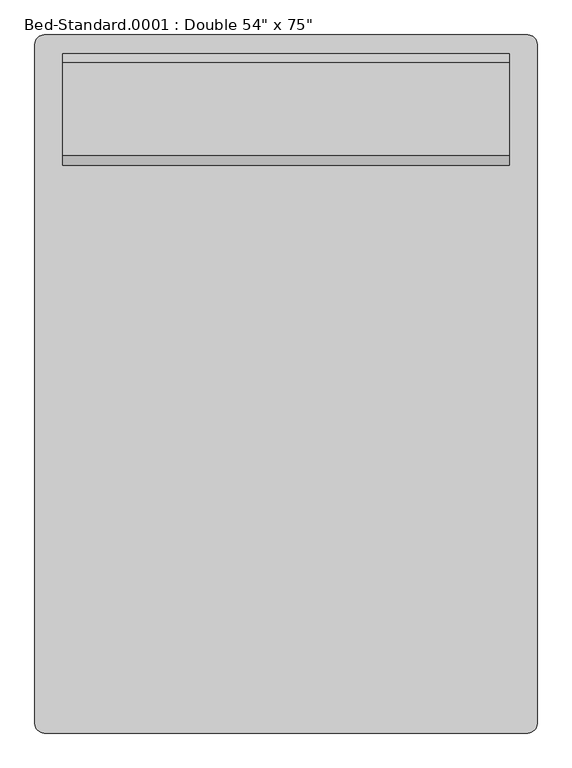
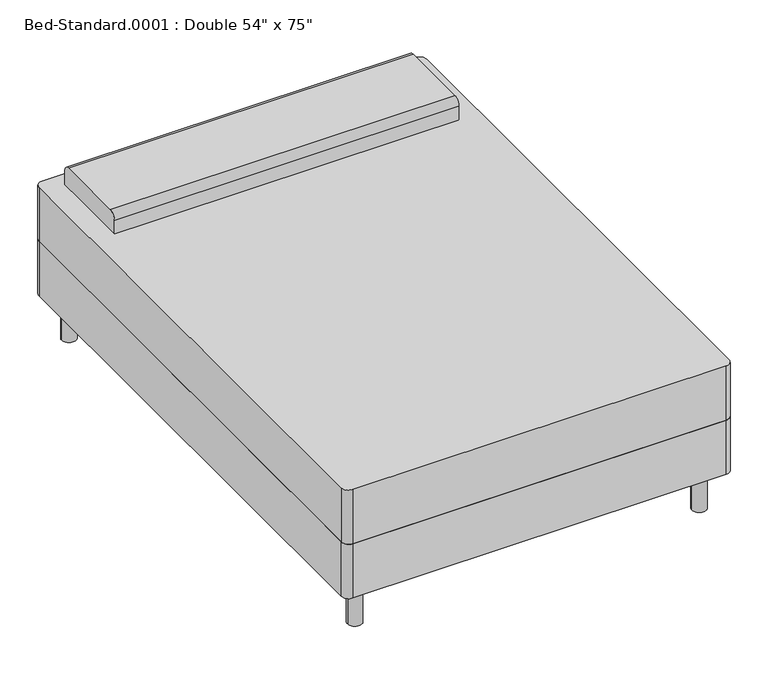
"""IFC4 building model written with IfcOpenShell, lengths in millimetres: furniture geometry."""

from ifc_helpers import new_model, si_unit, point, frame, frame_2d, origin, origin_with_axes, place, context, project, spatial, polyline, circle_curve, trimmed, segment, composite_curve, outline, extrude, source, transform, mapped, element, save


def furniture_0253826f(model_context):
    return source(origin(), model_context, "Body", "SweptSolid", [
        extrude(outline(composite_curve([segment(polyline([(-414.3114754, -972.695082), (-414.3114754, 881.504918)]), True, "CONTINUOUS"), segment(trimmed(circle_curve(frame_2d((-388.9114754, 881.504918)), 25.4), [point((-414.3114754, 881.504918))], [point((-388.9114754, 906.904918))], False, "CARTESIAN"), True, "CONTINUOUS"), segment(polyline([(-388.9114754, 906.904918), (931.8885246, 906.904918)]), True, "CONTINUOUS"), segment(trimmed(circle_curve(frame_2d((931.8885246, 881.504918)), 25.4), [point((931.8885246, 906.904918))], [point((957.2885246, 881.504918))], False, "CARTESIAN"), True, "CONTINUOUS"), segment(polyline([(957.2885246, 881.504918), (957.2885246, -972.695082)]), True, "CONTINUOUS"), segment(trimmed(circle_curve(frame_2d((931.8885246, -972.695082)), 25.4), [point((957.2885246, -972.695082))], [point((931.8885246, -998.095082))], False, "CARTESIAN"), True, "CONTINUOUS"), segment(polyline([(931.8885246, -998.095082), (-388.9114754, -998.095082)]), True, "CONTINUOUS"), segment(trimmed(circle_curve(frame_2d((-388.9114754, -972.695082)), 25.4), [point((-388.9114754, -998.095082))], [point((-414.3114754, -972.695082))], False, "CARTESIAN"), True, "CONTINUOUS")], self_intersect=False)), frame((0.0, 0.0, 152.4), z_axis=(0.0, 0.0, 1.0), x_axis=(1.0, 0.0, 0.0)), (0.0, 0.0, 1.0), 203.2),
        extrude(outline(composite_curve([segment(polyline([(551.304918, 558.8), (551.304918, 609.6)]), True, "CONTINUOUS"), segment(trimmed(circle_curve(frame_2d((576.704918, 609.6)), 25.4), [point((551.304918, 609.6))], [point((576.704918, 635.0))], False, "CARTESIAN"), True, "CONTINUOUS"), segment(polyline([(576.704918, 635.0), (830.704918, 635.0)]), True, "CONTINUOUS"), segment(trimmed(circle_curve(frame_2d((830.704918, 609.6)), 25.4), [point((830.704918, 635.0))], [point((856.104918, 609.6))], False, "CARTESIAN"), True, "CONTINUOUS"), segment(polyline([(856.104918, 609.6), (856.104918, 558.8), (551.304918, 558.8)]), True, "CONTINUOUS")], self_intersect=False)), frame((-338.1114754, 0.0, 0.0), z_axis=(1.0, 0.0, 0.0), x_axis=(0.0, 1.0, 0.0)), (0.0, 0.0, 1.0), 1219.2),
        extrude(outline(composite_curve([segment(trimmed(circle_curve(frame_2d((-338.1114754, 830.704918)), 25.4), [point((-363.5114754, 830.704918))], [point((-312.7114754, 830.704918))], False, "CARTESIAN"), True, "CONTINUOUS"), segment(trimmed(circle_curve(frame_2d((-338.1114754, 830.704918)), 25.4), [point((-312.7114754, 830.704918))], [point((-363.5114754, 830.704918))], False, "CARTESIAN"), True, "CONTINUOUS")], self_intersect=False)), origin_with_axes(), (0.0, 0.0, 1.0), 152.4),
        extrude(outline(composite_curve([segment(trimmed(circle_curve(frame_2d((881.0885246, 830.704918)), 25.4), [point((855.6885246, 830.704918))], [point((906.4885246, 830.704918))], False, "CARTESIAN"), True, "CONTINUOUS"), segment(trimmed(circle_curve(frame_2d((881.0885246, 830.704918)), 25.4), [point((906.4885246, 830.704918))], [point((855.6885246, 830.704918))], False, "CARTESIAN"), True, "CONTINUOUS")], self_intersect=False)), origin_with_axes(), (0.0, 0.0, 1.0), 152.4),
        extrude(outline(composite_curve([segment(trimmed(circle_curve(frame_2d((881.0885246, -921.895082)), 25.4), [point((855.6885246, -921.895082))], [point((906.4885246, -921.895082))], False, "CARTESIAN"), True, "CONTINUOUS"), segment(trimmed(circle_curve(frame_2d((881.0885246, -921.895082)), 25.4), [point((906.4885246, -921.895082))], [point((855.6885246, -921.895082))], False, "CARTESIAN"), True, "CONTINUOUS")], self_intersect=False)), origin_with_axes(), (0.0, 0.0, 1.0), 152.4),
        extrude(outline(composite_curve([segment(trimmed(circle_curve(frame_2d((-338.1114754, -921.895082)), 25.4), [point((-363.5114754, -921.895082))], [point((-312.7114754, -921.895082))], False, "CARTESIAN"), True, "CONTINUOUS"), segment(trimmed(circle_curve(frame_2d((-338.1114754, -921.895082)), 25.4), [point((-312.7114754, -921.895082))], [point((-363.5114754, -921.895082))], False, "CARTESIAN"), True, "CONTINUOUS")], self_intersect=False)), origin_with_axes(), (0.0, 0.0, 1.0), 152.4),
        extrude(outline(composite_curve([segment(polyline([(-388.9114754, 906.904918), (931.8885246, 906.904918)]), True, "CONTINUOUS"), segment(trimmed(circle_curve(frame_2d((931.8885246, 881.504918)), 25.4), [point((931.8885246, 906.904918))], [point((957.2885246, 881.504918))], False, "CARTESIAN"), True, "CONTINUOUS"), segment(polyline([(957.2885246, 881.504918), (957.2885246, -972.695082)]), True, "CONTINUOUS"), segment(trimmed(circle_curve(frame_2d((931.8885246, -972.695082)), 25.4), [point((957.2885246, -972.695082))], [point((931.8885246, -998.095082))], False, "CARTESIAN"), True, "CONTINUOUS"), segment(polyline([(931.8885246, -998.095082), (-388.9114754, -998.095082)]), True, "CONTINUOUS"), segment(trimmed(circle_curve(frame_2d((-388.9114754, -972.695082)), 25.4), [point((-388.9114754, -998.095082))], [point((-414.3114754, -972.695082))], False, "CARTESIAN"), True, "CONTINUOUS"), segment(polyline([(-414.3114754, -972.695082), (-414.3114754, 881.504918)]), True, "CONTINUOUS"), segment(trimmed(circle_curve(frame_2d((-388.9114754, 881.504918)), 25.4), [point((-414.3114754, 881.504918))], [point((-388.9114754, 906.904918))], False, "CARTESIAN"), True, "CONTINUOUS")], self_intersect=False)), frame((0.0, 0.0, 355.6), z_axis=(0.0, 0.0, 1.0), x_axis=(1.0, 0.0, 0.0)), (0.0, 0.0, 1.0), 203.2),
    ])


if __name__ == "__main__":
    model = new_model("IFC4")
    model_context = context("Model", 3, world=origin())
    ifc_project = project(units=[si_unit("LENGTHUNIT", "METRE", prefix="MILLI")], contexts=[model_context])
    site = spatial("IfcSite", under=ifc_project)
    building = spatial("IfcBuilding", under=site)
    placement = place(None, origin())
    furniture_shape = furniture_0253826f(model_context)
    element("IfcFurniture", 1, ObjectType="Bed-Standard.0001 : Double 54\" x 75\"", at=placement, inside=building, context=model_context, shape_type="MappedRepresentation", body=[
        mapped(furniture_shape, transform((0.0, 0.0, 0.0), x_axis=(1.0, 0.0, 0.0), y_axis=(0.0, 1.0, 0.0), z_axis=(0.0, 0.0, 1.0))),
    ])
    save(model, "model.ifc")

# Revit data of these elements
# Type "Bed-Standard.0001 : Double 54\" x 75\""
#   Assembly Code = "E2020200"
#   Length = 6' - 3"
#   Width = 4' - 6"
#   Leg Material = Steel, Chrome Plated
#   Mattress Material = Pine
#   Default Elevation = 0
# Element 1 (IfcFurniture, "Bed-Standard.0001 : Double 54\" x 75\"")
#   Materials on its faces: "Linen, White", "Steel, Chrome Plated"
# Materials
#   "Steel, Chrome Plated": class "Metal", colour RGB 17 17 17, transparency 0, Description = "Chromiuim plated steel", Cost = 0
#   "Pine": class "Wood", colour RGB 223 192 134, transparency 0, Description = "Pinus Echinata", Cost = 0
#   "Linen, White": class "Textile", colour RGB 247 247 239, transparency 0, Description = "Linen, white", Cost = 0
